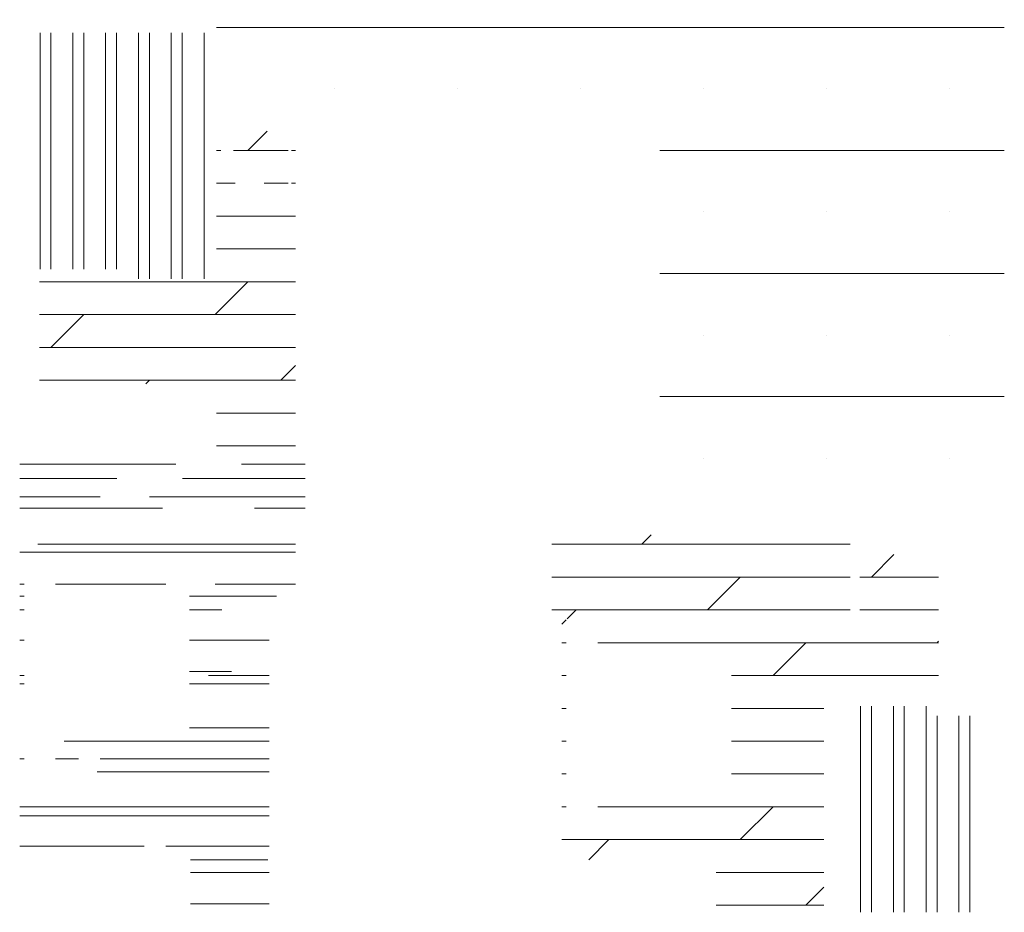
# Model space of a CAD drawing. Units: inches. Extents: x 111008 to 118198, y -138546 to -137723.
# Tile 1 of 4: x 111618 to 112068, y -138452 to -138044. Entities that reach past the tile are written whole.
import ezdxf

# ---------------------------------------------------------------- set-up
doc = ezdxf.new("R2010")
doc.units = ezdxf.units.IN
doc.header["$LTSCALE"] = 20
doc.header["$MEASUREMENT"] = 0
doc.layers.add('A-FLOR-PATT', color=251, linetype='Continuous', lineweight=9)
pattern_1 = [(270, (-148.02, 46.513), (15, -9e-16), []), (270, (-153.02, 41.513), (15, -9e-16), [])]
pattern_2 = [(0, (-148.02, 46.513), (0, 15), []), (45, (-148.02, 46.513), (-30, 30), [21.213203, -42.426407])]
pattern_3 = [(180, (-148.02, 46.513), (-1e-14, -56.25), []), (180, (-176.145, 74.64), (-1e-14, -56.25), [0, -56.25])]

msp = doc.modelspace()

# ---------------------------------------------------------------- hatches: boundary and pattern name
at = {"layer": 'A-FLOR-PATT'}
h = msp.add_hatch(dxfattribs=at)
h.set_pattern_fill('SACNCR', color=256, scale=600, angle=135)
h.set_pattern_definition(pattern_3)
h.paths.add_polyline_path([(112067.7, -138043.69), (111707.7, -138043.69), (111707.7, -138094.69), (111743.7, -138094.69), (111877.2, -138094.69), (111901.2, -138094.69), (111910.2, -138094.69), (112067.7, -138094.69)])
at = {"layer": 'A-FLOR-PATT', "ltscale": 0.5}
h = msp.add_hatch(dxfattribs=at)
h.set_pattern_fill('ANSI32', color=256, scale=40, angle=-135)
h.set_pattern_definition(pattern_1)
h.paths.add_polyline_path([(111703.2, -138049.69), (111617.7, -138049.69), (111617.7, -138085.69), (111617.7, -138157.69), (111670.2, -138157.69), (111670.2, -138162.19), (111703.2, -138162.19)])
at = {"layer": 'A-FLOR-PATT'}
h = msp.add_hatch(dxfattribs=at)
h.set_pattern_fill('DOLMIT', color=256, scale=60)
h.set_pattern_definition(pattern_2)
h.paths.add_polyline_path([(111743.7, -138162.19), (111626.7, -138162.19), (111626.7, -138210.13), (111707.7, -138210.13), (111707.7, -138234.19), (111707.7, -138238.69), (111743.7, -138238.69)])
h.paths.add_polyline_path([(111743.7, -138094.67), (111707.7, -138094.67), (111707.7, -138162.19), (111743.7, -138162.19)])
edge = h.paths.add_edge_path(flags=17)
edge.add_line((111707.7, -138094.69), (111743.7, -138094.69))
h.paths.add_polyline_path([(111741.96, -138130.19), (111741.96, -138097.18), (111740.47, -138097.18), (111740.47, -138130.19)], flags=16)
edge = h.paths.add_edge_path(flags=16)
edge.add_line((111741.27, -138094.69), (111743.7, -138094.69))
edge.add_line((111743.7, -138094.69), (111743.7, -138098.67))
edge.add_line((111743.7, -138098.67), (111741.96, -138098.67))
edge.add_line((111741.96, -138098.67), (111741.96, -138097.18))
edge.add_line((111741.96, -138097.18), (111740.72, -138097.18))
edge.add_line((111740.72, -138097.18), (111740.72, -138095.24))
edge.add_line((111740.72, -138095.24), (111740.86, -138095.24))
edge.add_line((111740.86, -138095.24), (111740.86, -138095.1))
edge.add_arc((111741.13, -138095.1), 0.275, 90, 180, ccw=False)
edge.add_line((111741.13, -138094.83), (111741.27, -138094.83))
edge.add_line((111741.27, -138094.83), (111741.27, -138094.69))
edge = h.paths.add_edge_path(flags=16)
edge.add_line((111710.13, -138094.69), (111707.7, -138094.69))
edge.add_line((111707.7, -138094.69), (111707.7, -138098.67))
edge.add_line((111707.7, -138098.67), (111709.44, -138098.67))
edge.add_line((111709.44, -138098.67), (111709.44, -138097.18))
edge.add_line((111709.44, -138097.18), (111710.68, -138097.18))
edge.add_line((111710.68, -138097.18), (111710.68, -138095.24))
edge.add_line((111710.68, -138095.24), (111710.54, -138095.24))
edge.add_line((111710.54, -138095.24), (111710.54, -138095.1))
edge.add_arc((111710.27, -138095.1), 0.275, 0, 90)
edge.add_line((111710.27, -138094.83), (111710.13, -138094.83))
edge.add_line((111710.13, -138094.83), (111710.13, -138094.69))
edge = h.paths.add_edge_path(flags=16)
edge.add_arc((111740.5, -138099.07), 31.12, 176.5003, 269.9437)
h = msp.add_hatch(dxfattribs=at)
h.set_pattern_fill('SACNCR', color=256, scale=600, angle=135)
h.set_pattern_definition(pattern_3)
h.paths.add_polyline_path([(112067.7, -138094.69), (111910.2, -138094.69), (111910.2, -138111.23), (111910.2, -138159.15), (111910.2, -138210.19), (111910.18, -138270.19), (112067.7, -138270.19)])
h = msp.add_hatch(dxfattribs=at)
h.set_pattern_fill('AR-RROOF', color=256, scale=30, angle=180)
h.set_pattern_definition([(180, (-148.02, 46.513), (-66, -30), [450, -60, 150, -30]), (180, (-187.92, 31.513), (30, -39.9), [90, -9.9, 180, -22.5]), (180, (-163.02, 21.013), (-156, -20.1), [240, -42, 120, -30])])
h.paths.add_polyline_path([(111743.7, -138274.69), (111748.2, -138274.69), (111748.2, -138238.69), (111743.7, -138238.69), (111707.7, -138238.69), (111617.7, -138238.69), (111617.7, -138274.69), (111617.7, -138427.63), (111695.7, -138427.63), (111695.7, -138451.69), (111731.7, -138451.69), (111731.7, -138312.52, -0.414214), (111737.7, -138306.52), (111743.7, -138306.52)])
h.paths.add_polyline_path([(111695.3, -138306.82), (111695.3, -138371.56), (111634.13, -138371.56), (111634.13, -138388.51), (111619.7, -138388.51), (111619.7, -138371.56), (111619.7, -138306.82), (111619.7, -138289.87), (111634.13, -138289.87), (111634.13, -138306.82)], flags=16)
edge = h.paths.add_edge_path(flags=0)
edge.add_line((111693.47, -138308.56), (111693.47, -138369.78))
edge.add_line((111693.47, -138369.78), (111650.08, -138369.78))
edge.add_ellipse((111663.67, -138377.01), major_axis=(-0.72, 20.39), ratio=0.705545, start_angle=59.9505, end_angle=60.0685)
edge.add_line((111650.07, -138369.81), (111650.07, -138369.78))
edge.add_line((111650.07, -138369.78), (111620.43, -138369.78))
edge.add_line((111620.43, -138369.78), (111620.43, -138308.56))
edge.add_line((111620.43, -138308.56), (111693.47, -138308.56))
h.paths.add_polyline_path([(111712.7, -138241.92), (111745.71, -138241.92), (111745.71, -138240.43), (111712.7, -138240.43)], flags=16)
h.paths.add_polyline_path([(111637.72, -138365.92), (111624.08, -138365.92), (111624.08, -138341.73), (111637.72, -138341.73), (111637.72, -138337.96), (111624.08, -138337.96), (111624.08, -138313.77), (111637.72, -138313.77)], flags=0)
h = msp.add_hatch(dxfattribs=at)
h.set_pattern_fill('DOLMIT', color=256, scale=60)
h.set_pattern_definition(pattern_2)
h.paths.add_polyline_path([(111997.2, -138279.19), (111860.94, -138279.19), (111860.94, -138315.21), (111865.44, -138315.21), (111865.44, -138427.63), (111935.94, -138427.63), (111935.94, -138451.69), (111985.2, -138451.69), (111985.2, -138351.21, -0.414214), (111988.2, -138348.21), (111997.2, -138348.21), (111997.2, -138315.21)])
h.paths.add_polyline_path([(111943.04, -138334.65), (111943.04, -138399.38), (111881.87, -138399.38), (111881.87, -138414.77), (111867.44, -138414.77), (111867.44, -138399.38), (111867.44, -138334.65), (111867.44, -138317.52), (111881.87, -138317.52), (111881.87, -138334.65)], flags=16)
edge = h.paths.add_edge_path(flags=0)
edge.add_line((111941.22, -138336.39), (111941.22, -138397.61))
edge.add_line((111941.22, -138397.61), (111897.82, -138397.61))
edge.add_ellipse((111911.41, -138404.84), major_axis=(-0.72, 20.39), ratio=0.705545, start_angle=59.9505, end_angle=60.0685)
edge.add_line((111897.81, -138397.64), (111897.81, -138397.61))
edge.add_line((111897.81, -138397.61), (111868.17, -138397.61))
edge.add_line((111868.17, -138397.61), (111868.17, -138336.39))
edge.add_line((111868.17, -138336.39), (111941.22, -138336.39))
h.paths.add_polyline_path([(111896.45, -138282.42), (111863.43, -138282.42), (111863.43, -138280.93), (111896.45, -138280.93)], flags=16)
h.paths.add_polyline_path([(111885.46, -138393.74), (111871.83, -138393.74), (111871.83, -138369.56), (111885.46, -138369.56), (111885.46, -138365.79), (111871.83, -138365.79), (111871.83, -138341.6), (111885.46, -138341.6)], flags=0)
h = msp.add_hatch(dxfattribs=at)
h.set_pattern_fill('DOLMIT', color=256, scale=60)
h.set_pattern_definition(pattern_2)
h.paths.add_polyline_path([(112037.64, -138288.19), (112001.7, -138288.19), (112001.7, -138315.21), (111997.2, -138315.21), (111997.2, -138348.21), (112001.7, -138348.21), (112001.7, -138357.44), (112037.64, -138357.44)])
at = {"layer": 'A-FLOR-PATT', "ltscale": 0.5}
h = msp.add_hatch(dxfattribs=at)
h.set_pattern_fill('ANSI32', color=256, scale=40, angle=-135)
h.set_pattern_definition(pattern_1)
h.paths.add_polyline_path([(112061.7, -138361.94), (112034.7, -138361.94), (112034.7, -138357.44), (112001.7, -138357.44), (112001.7, -138451.69), (112061.7, -138451.69)])

doc.saveas('drawing.dxf')
